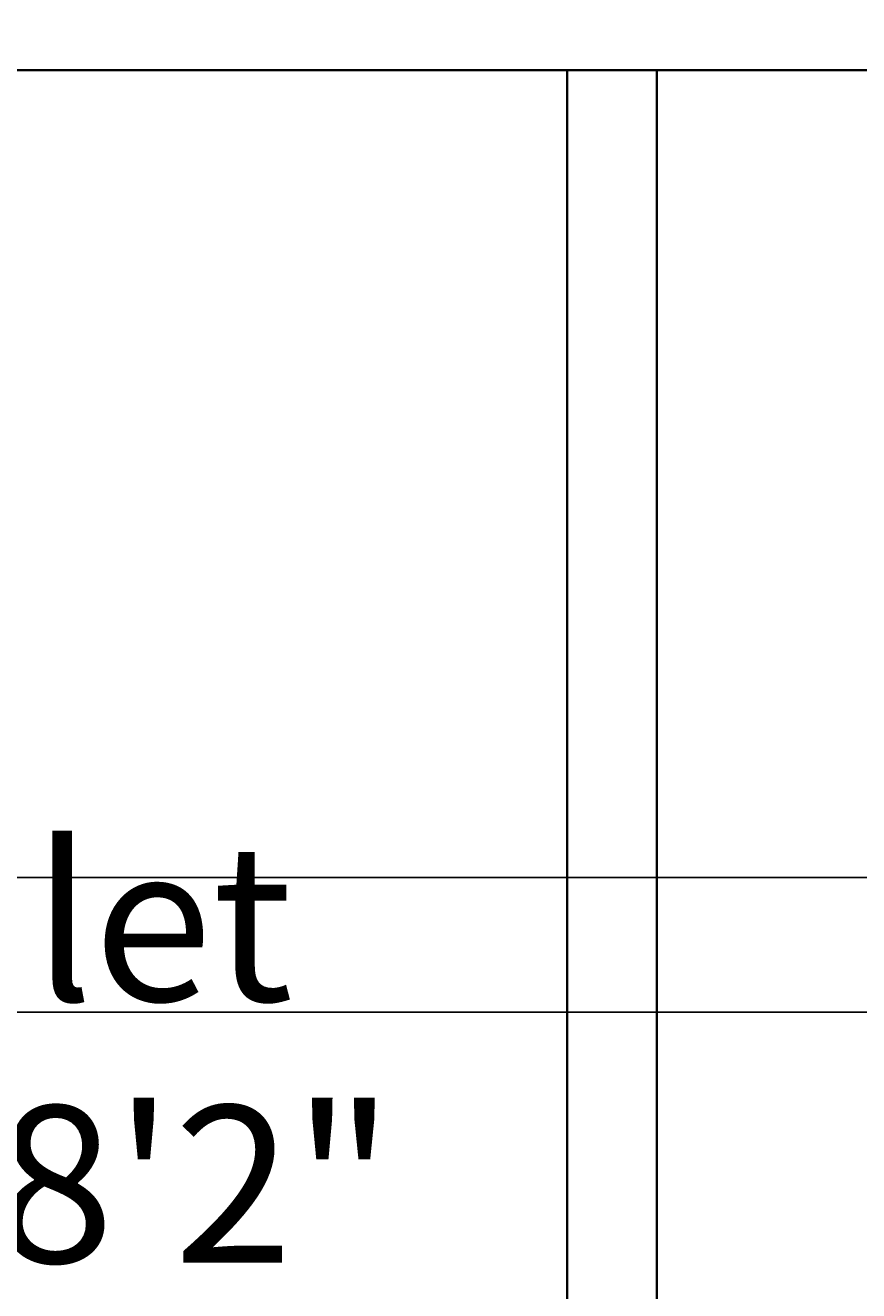
# Model space of a CAD drawing. Units: feet. Extents: x 105 to 1094, y -88 to 588.
# Tile 14 of 59: x 399 to 436, y 194 to 250. Entities that reach past the tile are written whole.
import ezdxf

# ---------------------------------------------------------------- set-up
doc = ezdxf.new("R2010")
doc.units = ezdxf.units.FT
doc.header["$MEASUREMENT"] = 0
for name, color, linetype, lineweight in [('A-ANNO-DIMS', 2, 'Continuous', 18), ('A-AREA-IDEN', 7, 'Continuous', 18), ('A-WALL', 7, 'Continuous', 35)]:
    doc.layers.add(name, color=color, linetype=linetype, lineweight=lineweight)
doc.styles.get("Standard").update_dxf_attribs({"font": 'arial.ttf'})
doc.dimstyles.get("Standard").update_dxf_attribs({"dimtxt": 0.18, "dimasz": 0.18, "dimexe": 0.18, "dimexo": 0.0625, "dimgap": 0.09, "dimtad": 0, "dimtih": 1, "dimtoh": 1, "dimdec": 4, "dimzin": 0, "dimdsep": 46, "dimtxsty": 'Standard', "dimcen": 0.09, "dimadec": 0, "dimazin": 0, "dimtfac": 1, "dimtdec": 4, "dimtofl": 0, "dimtmove": 0, "dimatfit": 3, "dimfxl": 1, "dimtolj": 1, "dimtzin": 0, "dimarcsym": 0})

# ---------------------------------------------------------------- blocks, each defined once
blk = doc.blocks.new('*D20')
at = {"layer": 'A-ANNO-DIMS', "color": 0, "lineweight": -2, "transparency": 16777216}
for p, q in [((150.688, 276.019), (150.688, -88.149)), ((1048.688, 276.019), (1048.688, -88.149)), ((150.868, -87.969), (599.399, -87.969)), ((1048.508, -87.969), (599.977, -87.969))]:
    blk.add_line(p, q, dxfattribs=at)
at = {"layer": 'A-ANNO-DIMS', "color": 0, "transparency": 16777216}
for points in [[(150.868, -87.939), (150.868, -87.999), (150.688, -87.969)], [(1048.508, -87.939), (1048.508, -87.999), (1048.688, -87.969)]]:
    blk.add_solid(points, dxfattribs=at)
at = {"layer": 'Defpoints', "color": 0, "transparency": 16777216}
for p in [(150.688, 276.081), (1048.688, 276.081), (1048.688, -87.969)]:
    blk.add_point(p, dxfattribs=at)
at = {"layer": 'A-ANNO-DIMS', "color": 0, "transparency": 16777216, "insert": (599.688, -87.969), "char_height": 0.18, "attachment_point": 5}
blk.add_mtext('\\A1;898', dxfattribs=at)
blk = doc.blocks.new('*D21')
at = {"layer": 'A-ANNO-DIMS', "color": 0, "lineweight": -2, "transparency": 16777216}
for p, q in [((849.626, 543.081), (105.458, 543.081)), ((105.638, 542.901), (105.638, 250.263)), ((105.638, -42.739), (105.638, 249.899)), ((849.626, -42.919), (105.458, -42.919))]:
    blk.add_line(p, q, dxfattribs=at)
at = {"layer": 'A-ANNO-DIMS', "color": 0, "transparency": 16777216}
for points in [[(105.608, 542.901), (105.668, 542.901), (105.638, 543.081)], [(105.608, -42.739), (105.668, -42.739), (105.638, -42.919)]]:
    blk.add_solid(points, dxfattribs=at)
at = {"layer": 'Defpoints', "color": 0, "transparency": 16777216}
for p in [(105.638, 543.081), (849.688, 543.081), (849.688, -42.919)]:
    blk.add_point(p, dxfattribs=at)
at = {"layer": 'A-ANNO-DIMS', "color": 0, "transparency": 16777216, "insert": (105.638, 250.081), "char_height": 0.18, "attachment_point": 5}
blk.add_mtext('\\A1;586', dxfattribs=at)
blk = doc.blocks.new('*D36')
at = {"layer": 'A-ANNO-DIMS', "color": 0, "lineweight": -2, "transparency": 16777216}
for p, q in [((547.235, 248.081), (105.458, 248.081)), ((105.638, 247.901), (105.638, 230.263)), ((105.638, 212.261), (105.638, 229.899)), ((546.626, 212.081), (105.458, 212.081))]:
    blk.add_line(p, q, dxfattribs=at)
at = {"layer": 'A-ANNO-DIMS', "color": 0, "transparency": 16777216}
for points in [[(105.608, 247.901), (105.668, 247.901), (105.638, 248.081)], [(105.608, 212.261), (105.668, 212.261), (105.638, 212.081)]]:
    blk.add_solid(points, dxfattribs=at)
at = {"layer": 'Defpoints', "color": 0, "transparency": 16777216}
for p in [(105.638, 248.081), (547.298, 248.081), (546.688, 212.081)]:
    blk.add_point(p, dxfattribs=at)
at = {"layer": 'A-ANNO-DIMS', "color": 0, "transparency": 16777216, "insert": (105.638, 230.081), "char_height": 0.18, "attachment_point": 5}
blk.add_mtext('\\A1;36', dxfattribs=at)
blk = doc.blocks.new('*D46')
at = {"layer": 'A-ANNO-DIMS', "color": 0, "lineweight": -2, "transparency": 16777216}
for p, q in [((580.626, 206.081), (105.458, 206.081)), ((105.638, 205.901), (105.638, 173.263)), ((105.638, 140.261), (105.638, 172.899)), ((580.626, 140.081), (105.458, 140.081))]:
    blk.add_line(p, q, dxfattribs=at)
at = {"layer": 'A-ANNO-DIMS', "color": 0, "transparency": 16777216}
for points in [[(105.608, 205.901), (105.668, 205.901), (105.638, 206.081)], [(105.608, 140.261), (105.668, 140.261), (105.638, 140.081)]]:
    blk.add_solid(points, dxfattribs=at)
at = {"layer": 'Defpoints', "color": 0, "transparency": 16777216}
for p in [(580.688, 206.081), (105.638, 140.081), (580.688, 140.081)]:
    blk.add_point(p, dxfattribs=at)
at = {"layer": 'A-ANNO-DIMS', "color": 0, "transparency": 16777216, "insert": (105.638, 173.081), "char_height": 0.18, "attachment_point": 5}
blk.add_mtext('\\A1;66', dxfattribs=at)

msp = doc.modelspace()

# ---------------------------------------------------------------- linework, layer by layer
at = {"layer": 'A-WALL'}
for p, q in [((552.6883, 248.0812), (370.6883, 248.0812)), ((422.6883, 248.0812), (370.6883, 248.0812)), ((422.6883, 248.0812), (422.6883, 150.0812)), ((552.6883, 248.0812), (426.6883, 248.0812)), ((426.6883, 248.0812), (426.6883, 146.0812))]:
    msp.add_line(p, q, dxfattribs=at)

# ---------------------------------------------------------------- texts
at = {"layer": 'A-AREA-IDEN', "insert": (446.7646, 194.9029), "char_height": 7, "attachment_point": 9}
msp.add_mtext_dynamic_manual_height_columns('\\pxqc;Toilet \\P4\' x 8\'2"', width=98.34246, gutter_width=1, heights=[0], dxfattribs=at)

# ---------------------------------------------------------------- dimensions: what is measured, and where the dimension line sits
at = {"layer": 'A-ANNO-DIMS'}
for base, p1, p2, picture, middle in [((105.6383, 543.0812), (849.6883, -42.9188), (849.6883, 543.0812), '*D21', (105.6383, 250.0812)), ((105.6383, 248.0812), (546.6883, 212.0812), (547.2975, 248.0812), '*D36', (105.6383, 230.0812)), ((105.6383, 140.0812), (580.6883, 206.0812), (580.6883, 140.0812), '*D46', (105.6383, 173.0812))]:
    dim = msp.add_linear_dim(base=base, p1=p1, p2=p2, angle=90, dimstyle='Standard', override={"dimdec": 0, "dimlfac": 1, "dimrnd": 0, "dimzin": 0, "dimdsep": 46, "dimlunit": 2}, dxfattribs=at)
    dim.commit()
    dim.dimension.update_dxf_attribs({"geometry": picture, "text_midpoint": middle})
dim = msp.add_linear_dim(base=(1048.6883, -87.9688), p1=(150.6883, 276.0812), p2=(1048.6883, 276.0812), dimstyle='Standard', override={"dimdec": 0, "dimlfac": 1, "dimrnd": 0, "dimzin": 0, "dimdsep": 46, "dimlunit": 2}, dxfattribs=at)
dim.commit()
dim.dimension.update_dxf_attribs({"geometry": '*D20', "text_midpoint": (599.6883, -87.9688)})

doc.saveas('drawing.dxf')
